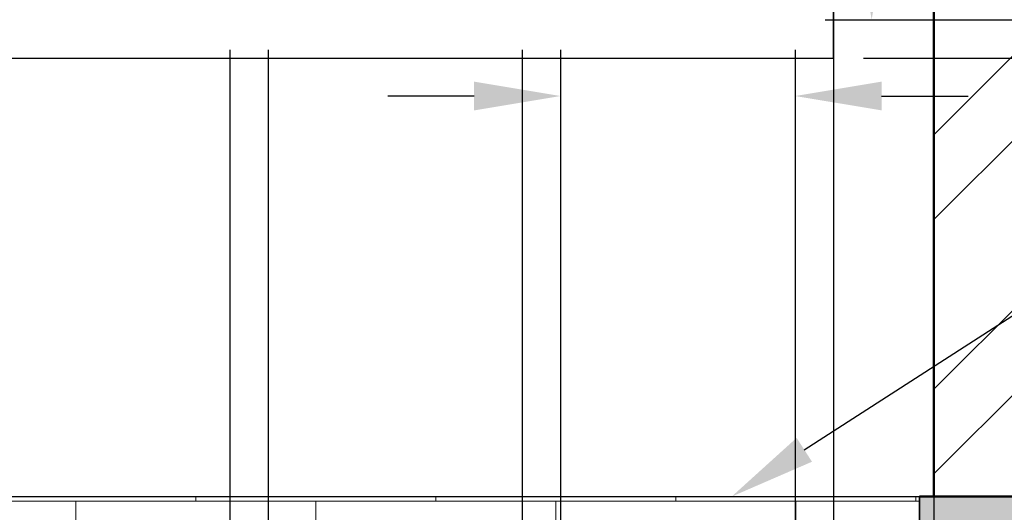
# Model space of a CAD drawing. Units: metres. Extents: x 22.1 to 34.4, y 4.4 to 12.4.
# Tile 5 of 8: x 29.6 to 31.7, y 8.5 to 9.5. Entities that reach past the tile are written whole.
import ezdxf
from ezdxf import colors
from ezdxf.entities.mleader import LeaderData, LeaderLine
from ezdxf.math import Vec2, Vec3

# ---------------------------------------------------------------- set-up
doc = ezdxf.new("R2010")
doc.units = ezdxf.units.M
doc.header["$MEASUREMENT"] = 0
for name, color, linetype, lineweight in [('A-ANNO-DIMS', 2, 'Continuous', 18), ('A-ANNO-TEXT', 7, 'Continuous', 18), ('A-FLOR', 3, 'Continuous', 25), ('A-FLOR-PATT', 252, 'Continuous', 13), ('A-GLAZ', 4, 'Continuous', 25), ('A-WALL', 7, 'Continuous', 50), ('A-WALL-PATT', 8, 'Continuous', 18), ('S-FNDN', 1, 'Continuous', 35), ('S-SLAB-PATT', 8, 'Continuous', 13)]:
    doc.layers.add(name, color=color, linetype=linetype, lineweight=lineweight)
doc.styles.get("Standard").update_dxf_attribs({"font": 'arial.ttf'})
doc.dimstyles.get("Standard").update_dxf_attribs({"dimtxt": 0.18, "dimasz": 0.18, "dimexe": 0.18, "dimexo": 0.0625, "dimgap": 0.09, "dimtad": 0, "dimtih": 1, "dimtoh": 1, "dimzin": 0, "dimdsep": 46, "dimtxsty": 'Standard', "dimcen": 0.09, "dimadec": 0, "dimazin": 0, "dimtfac": 1, "dimtofl": 0, "dimtmove": 0, "dimatfit": 3, "dimfxl": 1, "dimtolj": 1, "dimtzin": 0, "dimarcsym": 0})

# ---------------------------------------------------------------- blocks, each defined once
blk = doc.blocks.new('*D18')
at = {"layer": 'A-ANNO-DIMS', "color": 0, "lineweight": -2, "transparency": 16777216}
for p, q in [((31.3118, 10.5649), (31.5885, 10.5649)), ((31.4085, 10.3849), (31.4085, 10.2175)), ((31.4085, 9.6839), (31.4085, 9.8513)), ((31.3118, 9.5039), (31.5885, 9.5039))]:
    blk.add_line(p, q, dxfattribs=at)
at = {"layer": 'A-ANNO-DIMS', "color": 0, "transparency": 16777216}
for points in [[(31.3785, 10.3849), (31.4385, 10.3849), (31.4085, 10.5649)], [(31.3785, 9.6839), (31.4385, 9.6839), (31.4085, 9.5039)]]:
    blk.add_solid(points, dxfattribs=at)
at = {"layer": 'Defpoints', "color": 0, "transparency": 16777216}
for p in [(31.2493, 10.5649), (31.4085, 10.5649), (31.2493, 9.5039)]:
    blk.add_point(p, dxfattribs=at)
at = {"layer": 'A-ANNO-DIMS', "color": 0, "transparency": 16777216, "insert": (31.4085, 10.0344), "char_height": 0.18, "attachment_point": 5}
blk.add_mtext('\\A1;WINDOW PANE 490 1.06 TYP.', dxfattribs=at)
blk = doc.blocks.new('*D19')
at = {"layer": 'A-ANNO-DIMS', "color": 0, "lineweight": -2, "transparency": 16777216}
for p, q in [((30.7603, 9.4414), (30.7603, 9.1648)), ((31.2493, 9.4414), (31.2493, 9.1648)), ((30.5803, 9.3448), (30.4003, 9.3448)), ((31.4293, 9.3448), (31.6093, 9.3448))]:
    blk.add_line(p, q, dxfattribs=at)
at = {"layer": 'A-ANNO-DIMS', "color": 0, "transparency": 16777216}
for points in [[(30.5803, 9.3748), (30.5803, 9.3148), (30.7603, 9.3448)], [(31.4293, 9.3748), (31.4293, 9.3148), (31.2493, 9.3448)]]:
    blk.add_solid(points, dxfattribs=at)
at = {"layer": 'Defpoints', "color": 0, "transparency": 16777216}
for p in [(30.7603, 9.5039), (31.2493, 9.5039), (31.2493, 9.3448)]:
    blk.add_point(p, dxfattribs=at)
at = {"layer": 'A-ANNO-DIMS', "color": 0, "transparency": 16777216, "insert": (32.2423, 9.3448), "char_height": 0.18, "attachment_point": 5}
blk.add_mtext('\\A1;0.49 TYP.', dxfattribs=at)
blk = doc.blocks.new('*D20')
at = {"layer": 'A-ANNO-DIMS', "color": 0, "lineweight": -2, "transparency": 16777216}
for p, q in [((29.4798, 10.5649), (29.2032, 10.5649)), ((29.3832, 10.3849), (29.3832, 10.2176)), ((29.3832, 9.6839), (29.3832, 9.8512)), ((29.4798, 9.5039), (29.2032, 9.5039))]:
    blk.add_line(p, q, dxfattribs=at)
at = {"layer": 'A-ANNO-DIMS', "color": 0, "transparency": 16777216}
for points in [[(29.3532, 10.3849), (29.4132, 10.3849), (29.3832, 10.5649)], [(29.3532, 9.6839), (29.4132, 9.6839), (29.3832, 9.5039)]]:
    blk.add_solid(points, dxfattribs=at)
at = {"layer": 'Defpoints', "color": 0, "transparency": 16777216}
for p in [(29.3832, 10.5649), (29.5423, 10.5649), (29.5423, 9.5039)]:
    blk.add_point(p, dxfattribs=at)
at = {"layer": 'A-ANNO-DIMS', "color": 0, "transparency": 16777216, "insert": (29.3832, 10.0344), "char_height": 0.18, "attachment_point": 5}
blk.add_mtext('\\A1;WINDOW PANE 530 1.06 TYP.', dxfattribs=at)
blk = doc.blocks.new('*D23')
at = {"layer": 'A-ANNO-DIMS', "color": 0, "lineweight": -2, "transparency": 16777216}
for p, q in [((28.0901, 11.4474), (28.0901, 6.2449)), ((31.5381, 11.4474), (31.5381, 6.2449)), ((28.2701, 6.4249), (29.4202, 6.4249)), ((31.3581, 6.4249), (30.2079, 6.4249))]:
    blk.add_line(p, q, dxfattribs=at)
at = {"layer": 'A-ANNO-DIMS', "color": 0, "transparency": 16777216}
for points in [[(28.2701, 6.4549), (28.2701, 6.3949), (28.0901, 6.4249)], [(31.3581, 6.4549), (31.3581, 6.3949), (31.5381, 6.4249)]]:
    blk.add_solid(points, dxfattribs=at)
at = {"layer": 'Defpoints', "color": 0, "transparency": 16777216}
for p in [(28.0901, 11.5099), (31.5381, 11.5099), (31.5381, 6.4249)]:
    blk.add_point(p, dxfattribs=at)
at = {"layer": 'A-ANNO-DIMS', "color": 0, "transparency": 16777216, "insert": (29.8141, 6.4249), "char_height": 0.18, "attachment_point": 5}
blk.add_mtext('\\A1;3.448', dxfattribs=at)
blk = doc.blocks.new('*D27')
at = {"layer": 'A-ANNO-DIMS', "color": 0, "lineweight": -2, "transparency": 16777216}
for p, q in [((31.5381, 11.4474), (31.5381, 6.2449)), ((31.7781, 11.4474), (31.7781, 6.2449)), ((31.3581, 6.4249), (31.1781, 6.4249)), ((31.9581, 6.4249), (32.1381, 6.4249))]:
    blk.add_line(p, q, dxfattribs=at)
at = {"layer": 'A-ANNO-DIMS', "color": 0, "transparency": 16777216}
for points in [[(31.3581, 6.4549), (31.3581, 6.3949), (31.5381, 6.4249)], [(31.9581, 6.4549), (31.9581, 6.3949), (31.7781, 6.4249)]]:
    blk.add_solid(points, dxfattribs=at)
at = {"layer": 'Defpoints', "color": 0, "transparency": 16777216}
for p in [(31.5381, 11.5099), (31.7781, 11.5099), (31.7781, 6.4249)]:
    blk.add_point(p, dxfattribs=at)
at = {"layer": 'A-ANNO-DIMS', "color": 0, "transparency": 16777216, "insert": (32.4615, 6.4249), "char_height": 0.18, "attachment_point": 5}
blk.add_mtext('\\A1;0.24', dxfattribs=at)
blk = doc.blocks.new('*D28')
at = {"layer": 'A-ANNO-DIMS', "color": 0, "lineweight": -2, "transparency": 16777216}
for p, q in [((31.7781, 11.4474), (31.7781, 6.2449)), ((31.9781, 11.4474), (31.9781, 6.2449)), ((31.5981, 6.4249), (31.4181, 6.4249)), ((32.1581, 6.4249), (32.3381, 6.4249))]:
    blk.add_line(p, q, dxfattribs=at)
at = {"layer": 'A-ANNO-DIMS', "color": 0, "transparency": 16777216}
for points in [[(31.5981, 6.4549), (31.5981, 6.3949), (31.7781, 6.4249)], [(32.1581, 6.4549), (32.1581, 6.3949), (31.9781, 6.4249)]]:
    blk.add_solid(points, dxfattribs=at)
at = {"layer": 'Defpoints', "color": 0, "transparency": 16777216}
for p in [(31.7781, 11.5099), (31.9781, 11.5099), (31.9781, 6.4249)]:
    blk.add_point(p, dxfattribs=at)
at = {"layer": 'A-ANNO-DIMS', "color": 0, "transparency": 16777216, "insert": (32.6615, 6.4249), "char_height": 0.18, "attachment_point": 5}
blk.add_mtext('\\A1;0.20', dxfattribs=at)
blk = doc.blocks.new('*D33')
at = {"layer": 'A-ANNO-DIMS', "color": 0, "lineweight": -2, "transparency": 16777216}
for p, q in [((31.5381, 11.4474), (31.5381, 6.2449)), ((31.3293, 10.5774), (31.3293, 6.2449)), ((31.1493, 6.4249), (30.9693, 6.4249)), ((31.7181, 6.4249), (31.8981, 6.4249))]:
    blk.add_line(p, q, dxfattribs=at)
at = {"layer": 'A-ANNO-DIMS', "color": 0, "transparency": 16777216}
for points in [[(31.1493, 6.4549), (31.1493, 6.3949), (31.3293, 6.4249)], [(31.7181, 6.4549), (31.7181, 6.3949), (31.5381, 6.4249)]]:
    blk.add_solid(points, dxfattribs=at)
at = {"layer": 'Defpoints', "color": 0, "transparency": 16777216}
for p in [(31.5381, 11.5099), (31.3293, 10.6399), (31.5381, 6.4249)]:
    blk.add_point(p, dxfattribs=at)
at = {"layer": 'A-ANNO-DIMS', "color": 0, "transparency": 16777216, "insert": (32.2045, 6.4249), "char_height": 0.18, "attachment_point": 5}
blk.add_mtext('\\A1;0.21', dxfattribs=at)
blk = doc.blocks.new('*D34')
at = {"layer": 'A-ANNO-DIMS', "color": 0, "lineweight": -2, "transparency": 16777216}
for p, q in [((28.8933, 9.3614), (28.8933, 6.2449)), ((31.3293, 9.3614), (31.3293, 6.2449)), ((29.0733, 6.4249), (29.7162, 6.4249)), ((31.1493, 6.4249), (30.5065, 6.4249))]:
    blk.add_line(p, q, dxfattribs=at)
at = {"layer": 'A-ANNO-DIMS', "color": 0, "transparency": 16777216}
for points in [[(29.0733, 6.4549), (29.0733, 6.3949), (28.8933, 6.4249)], [(31.1493, 6.4549), (31.1493, 6.3949), (31.3293, 6.4249)]]:
    blk.add_solid(points, dxfattribs=at)
at = {"layer": 'Defpoints', "color": 0, "transparency": 16777216}
for p in [(28.8933, 9.4239), (31.3293, 9.4239), (31.3293, 6.4249)]:
    blk.add_point(p, dxfattribs=at)
at = {"layer": 'A-ANNO-DIMS', "color": 0, "transparency": 16777216, "insert": (30.1113, 6.4249), "char_height": 0.18, "attachment_point": 5}
blk.add_mtext('\\A1;2.436', dxfattribs=at)
blk = doc.blocks.new('*D35')
at = {"layer": 'A-ANNO-DIMS', "color": 0, "lineweight": -2, "transparency": 16777216}
for p, q in [((28.9733, 9.4414), (28.9733, 6.2449)), ((28.8933, 9.3614), (28.8933, 6.2449)), ((28.7133, 6.4249), (28.5333, 6.4249)), ((29.1533, 6.4249), (29.3333, 6.4249))]:
    blk.add_line(p, q, dxfattribs=at)
at = {"layer": 'A-ANNO-DIMS', "color": 0, "transparency": 16777216}
for points in [[(28.7133, 6.4549), (28.7133, 6.3949), (28.8933, 6.4249)], [(29.1533, 6.4549), (29.1533, 6.3949), (28.9733, 6.4249)]]:
    blk.add_solid(points, dxfattribs=at)
at = {"layer": 'Defpoints', "color": 0, "transparency": 16777216}
for p in [(28.9733, 9.5039), (28.8933, 9.4239), (28.9733, 6.4249)]:
    blk.add_point(p, dxfattribs=at)
at = {"layer": 'A-ANNO-DIMS', "color": 0, "transparency": 16777216, "insert": (29.6573, 6.4249), "char_height": 0.18, "attachment_point": 5}
blk.add_mtext('\\A1;0.08', dxfattribs=at)
blk = doc.blocks.new('*D36')
at = {"layer": 'A-ANNO-DIMS', "color": 0, "lineweight": -2, "transparency": 16777216}
for p, q in [((29.4623, 9.4414), (29.4623, 6.2449)), ((29.5423, 9.4414), (29.5423, 6.2449)), ((29.2823, 6.4249), (29.1023, 6.4249)), ((29.7223, 6.4249), (29.9023, 6.4249))]:
    blk.add_line(p, q, dxfattribs=at)
at = {"layer": 'A-ANNO-DIMS', "color": 0, "transparency": 16777216}
for points in [[(29.2823, 6.4549), (29.2823, 6.3949), (29.4623, 6.4249)], [(29.7223, 6.4549), (29.7223, 6.3949), (29.5423, 6.4249)]]:
    blk.add_solid(points, dxfattribs=at)
at = {"layer": 'Defpoints', "color": 0, "transparency": 16777216}
for p in [(29.4623, 9.5039), (29.5423, 9.5039), (29.5423, 6.4249)]:
    blk.add_point(p, dxfattribs=at)
at = {"layer": 'A-ANNO-DIMS', "color": 0, "transparency": 16777216, "insert": (30.2263, 6.4249), "char_height": 0.18, "attachment_point": 5}
blk.add_mtext('\\A1;0.08', dxfattribs=at)
blk = doc.blocks.new('*D37')
at = {"layer": 'A-ANNO-DIMS', "color": 0, "lineweight": -2, "transparency": 16777216}
for p, q in [((30.0713, 9.4414), (30.0713, 6.2449)), ((30.1513, 9.4414), (30.1513, 6.2449)), ((29.8913, 6.4249), (29.7113, 6.4249)), ((30.3313, 6.4249), (30.5113, 6.4249))]:
    blk.add_line(p, q, dxfattribs=at)
at = {"layer": 'A-ANNO-DIMS', "color": 0, "transparency": 16777216}
for points in [[(29.8913, 6.4549), (29.8913, 6.3949), (30.0713, 6.4249)], [(30.3313, 6.4549), (30.3313, 6.3949), (30.1513, 6.4249)]]:
    blk.add_solid(points, dxfattribs=at)
at = {"layer": 'Defpoints', "color": 0, "transparency": 16777216}
for p in [(30.0713, 9.5039), (30.1513, 9.5039), (30.1513, 6.4249)]:
    blk.add_point(p, dxfattribs=at)
at = {"layer": 'A-ANNO-DIMS', "color": 0, "transparency": 16777216, "insert": (30.8353, 6.4249), "char_height": 0.18, "attachment_point": 5}
blk.add_mtext('\\A1;0.08', dxfattribs=at)
blk = doc.blocks.new('*D38')
at = {"layer": 'A-ANNO-DIMS', "color": 0, "lineweight": -2, "transparency": 16777216}
for p, q in [((30.6803, 9.4414), (30.6803, 6.2449)), ((30.7603, 9.4414), (30.7603, 6.2449)), ((30.5003, 6.4249), (30.3203, 6.4249)), ((30.9403, 6.4249), (31.1203, 6.4249))]:
    blk.add_line(p, q, dxfattribs=at)
at = {"layer": 'A-ANNO-DIMS', "color": 0, "transparency": 16777216}
for points in [[(30.5003, 6.4549), (30.5003, 6.3949), (30.6803, 6.4249)], [(30.9403, 6.4549), (30.9403, 6.3949), (30.7603, 6.4249)]]:
    blk.add_solid(points, dxfattribs=at)
at = {"layer": 'Defpoints', "color": 0, "transparency": 16777216}
for p in [(30.6803, 9.5039), (30.7603, 9.5039), (30.7603, 6.4249)]:
    blk.add_point(p, dxfattribs=at)
at = {"layer": 'A-ANNO-DIMS', "color": 0, "transparency": 16777216, "insert": (31.4443, 6.4249), "char_height": 0.18, "attachment_point": 5}
blk.add_mtext('\\A1;0.08', dxfattribs=at)
blk = doc.blocks.new('*D39')
at = {"layer": 'A-ANNO-DIMS', "color": 0, "lineweight": -2, "transparency": 16777216}
for p, q in [((31.2493, 9.4414), (31.2493, 6.2449)), ((31.3293, 9.3614), (31.3293, 6.2449)), ((31.0693, 6.4249), (30.8893, 6.4249)), ((31.5093, 6.4249), (31.6893, 6.4249))]:
    blk.add_line(p, q, dxfattribs=at)
at = {"layer": 'A-ANNO-DIMS', "color": 0, "transparency": 16777216}
for points in [[(31.0693, 6.4549), (31.0693, 6.3949), (31.2493, 6.4249)], [(31.5093, 6.4549), (31.5093, 6.3949), (31.3293, 6.4249)]]:
    blk.add_solid(points, dxfattribs=at)
at = {"layer": 'Defpoints', "color": 0, "transparency": 16777216}
for p in [(31.2493, 9.5039), (31.3293, 9.4239), (31.3293, 6.4249)]:
    blk.add_point(p, dxfattribs=at)
at = {"layer": 'A-ANNO-DIMS', "color": 0, "transparency": 16777216, "insert": (32.0133, 6.4249), "char_height": 0.18, "attachment_point": 5}
blk.add_mtext('\\A1;0.08', dxfattribs=at)
blk = doc.blocks.new('*D40')
at = {"layer": 'A-ANNO-DIMS', "color": 0, "lineweight": -2, "transparency": 16777216}
for p, q in [((31.3918, 10.6399), (33.8537, 10.6399)), ((33.6737, 10.4599), (33.6737, 10.2138)), ((33.6737, 9.6039), (33.6737, 9.85)), ((31.3918, 9.4239), (33.8537, 9.4239))]:
    blk.add_line(p, q, dxfattribs=at)
at = {"layer": 'A-ANNO-DIMS', "color": 0, "transparency": 16777216}
for points in [[(33.6437, 10.4599), (33.7037, 10.4599), (33.6737, 10.6399)], [(33.6437, 9.6039), (33.7037, 9.6039), (33.6737, 9.4239)]]:
    blk.add_solid(points, dxfattribs=at)
at = {"layer": 'Defpoints', "color": 0, "transparency": 16777216}
for p in [(31.3293, 10.6399), (31.3293, 9.4239), (33.6737, 9.4239)]:
    blk.add_point(p, dxfattribs=at)
at = {"layer": 'A-ANNO-DIMS', "color": 0, "transparency": 16777216, "insert": (33.6737, 10.0319), "char_height": 0.18, "attachment_point": 5}
blk.add_mtext('\\A1;1.216', dxfattribs=at)
blk = doc.blocks.new('*D42')
at = {"layer": 'A-ANNO-DIMS', "color": 0, "lineweight": -2, "transparency": 16777216}
for p, q in [((33.6737, 9.6839), (33.6737, 9.8639)), ((33.6737, 9.8639), (33.8537, 9.8639)), ((31.3118, 9.5039), (33.8537, 9.5039)), ((31.3918, 9.4239), (33.8537, 9.4239)), ((33.6737, 9.2439), (33.6737, 9.0639))]:
    blk.add_line(p, q, dxfattribs=at)
at = {"layer": 'A-ANNO-DIMS', "color": 0, "transparency": 16777216}
for points in [[(33.6437, 9.6839), (33.7037, 9.6839), (33.6737, 9.5039)], [(33.6437, 9.2439), (33.7037, 9.2439), (33.6737, 9.4239)]]:
    blk.add_solid(points, dxfattribs=at)
at = {"layer": 'Defpoints', "color": 0, "transparency": 16777216}
for p in [(31.2493, 9.5039), (33.6737, 9.5039), (31.3293, 9.4239)]:
    blk.add_point(p, dxfattribs=at)
at = {"layer": 'A-ANNO-DIMS', "color": 0, "transparency": 16777216, "insert": (34.1776, 9.8639), "char_height": 0.18, "attachment_point": 5}
blk.add_mtext('\\A1;0.08', dxfattribs=at)
blk = doc.blocks.new('*D43')
at = {"layer": 'A-ANNO-DIMS', "color": 0, "lineweight": -2, "transparency": 16777216}
for p, q in [((31.3918, 9.4239), (33.8537, 9.4239)), ((33.6737, 9.2439), (33.6737, 9.1488)), ((33.6737, 8.6899), (33.6737, 8.785)), ((31.5706, 8.5099), (33.8537, 8.5099))]:
    blk.add_line(p, q, dxfattribs=at)
at = {"layer": 'A-ANNO-DIMS', "color": 0, "transparency": 16777216}
for points in [[(33.6437, 9.2439), (33.7037, 9.2439), (33.6737, 9.4239)], [(33.6437, 8.6899), (33.7037, 8.6899), (33.6737, 8.5099)]]:
    blk.add_solid(points, dxfattribs=at)
at = {"layer": 'Defpoints', "color": 0, "transparency": 16777216}
for p in [(31.3293, 9.4239), (31.5081, 8.5099), (33.6737, 8.5099)]:
    blk.add_point(p, dxfattribs=at)
at = {"layer": 'A-ANNO-DIMS', "color": 0, "transparency": 16777216, "insert": (33.6737, 8.9669), "char_height": 0.18, "attachment_point": 5}
blk.add_mtext('\\A1;0.914', dxfattribs=at)
blk = doc.blocks.new('*D44')
at = {"layer": 'A-ANNO-DIMS', "color": 0, "lineweight": -2, "transparency": 16777216}
for p, q in [((33.6737, 8.6899), (33.6737, 8.8699)), ((24.8474, 8.5099), (33.8537, 8.5099)), ((24.5474, 8.4099), (33.8537, 8.4099)), ((33.6737, 8.2299), (33.6737, 8.0499)), ((33.6737, 8.0499), (33.4937, 8.0499))]:
    blk.add_line(p, q, dxfattribs=at)
at = {"layer": 'A-ANNO-DIMS', "color": 0, "transparency": 16777216}
for points in [[(33.6437, 8.6899), (33.7037, 8.6899), (33.6737, 8.5099)], [(33.6437, 8.2299), (33.7037, 8.2299), (33.6737, 8.4099)]]:
    blk.add_solid(points, dxfattribs=at)
at = {"layer": 'Defpoints', "color": 0, "transparency": 16777216}
for p in [(24.7849, 8.5099), (24.4849, 8.4099), (33.6737, 8.4099)]:
    blk.add_point(p, dxfattribs=at)
at = {"layer": 'A-ANNO-DIMS', "color": 0, "transparency": 16777216, "insert": (33.1702, 8.0499), "char_height": 0.18, "attachment_point": 5}
blk.add_mtext('\\A1;0.10', dxfattribs=at)
blk = doc.blocks.new('*D45')
at = {"layer": 'A-ANNO-DIMS', "color": 0, "lineweight": -2, "transparency": 16777216}
for p, q in [((33.6737, 8.5899), (33.6737, 8.7699)), ((24.5474, 8.4099), (33.8537, 8.4099)), ((24.8474, 8.3119), (33.8537, 8.3119)), ((33.6737, 8.1319), (33.6737, 7.9519)), ((33.6737, 7.9519), (33.4937, 7.9519))]:
    blk.add_line(p, q, dxfattribs=at)
at = {"layer": 'A-ANNO-DIMS', "color": 0, "transparency": 16777216}
for points in [[(33.6437, 8.5899), (33.7037, 8.5899), (33.6737, 8.4099)], [(33.6437, 8.1319), (33.7037, 8.1319), (33.6737, 8.3119)]]:
    blk.add_solid(points, dxfattribs=at)
at = {"layer": 'Defpoints', "color": 0, "transparency": 16777216}
for p in [(24.4849, 8.4099), (24.7849, 8.3119), (33.6737, 8.3119)]:
    blk.add_point(p, dxfattribs=at)
at = {"layer": 'A-ANNO-DIMS', "color": 0, "transparency": 16777216, "insert": (33.0998, 7.9519), "char_height": 0.18, "attachment_point": 5}
blk.add_mtext('\\A1;0.098', dxfattribs=at)
blk = doc.blocks.new('*D46')
at = {"layer": 'A-ANNO-DIMS', "color": 0, "lineweight": -2, "transparency": 16777216}
for p, q in [((33.6737, 8.4919), (33.6737, 8.6719)), ((24.8474, 8.3119), (33.8537, 8.3119)), ((24.8474, 8.1578), (33.8537, 8.1578)), ((33.6737, 7.9778), (33.6737, 7.7978)), ((33.6737, 7.7978), (33.4937, 7.7978))]:
    blk.add_line(p, q, dxfattribs=at)
at = {"layer": 'A-ANNO-DIMS', "color": 0, "transparency": 16777216}
for points in [[(33.6437, 8.4919), (33.7037, 8.4919), (33.6737, 8.3119)], [(33.6437, 7.9778), (33.7037, 7.9778), (33.6737, 8.1578)]]:
    blk.add_solid(points, dxfattribs=at)
at = {"layer": 'Defpoints', "color": 0, "transparency": 16777216}
for p in [(24.7849, 8.3119), (24.7849, 8.1578), (33.6737, 8.1578)]:
    blk.add_point(p, dxfattribs=at)
at = {"layer": 'A-ANNO-DIMS', "color": 0, "transparency": 16777216, "insert": (33.1692, 7.7978), "char_height": 0.18, "attachment_point": 5}
blk.add_mtext('\\A1;0.15', dxfattribs=at)
blk = doc.blocks.new('*D47')
at = {"layer": 'A-ANNO-DIMS', "color": 0, "lineweight": -2, "transparency": 16777216}
for p, q in [((33.6737, 8.3378), (33.6737, 8.5178)), ((24.8474, 8.1578), (33.8537, 8.1578)), ((24.8474, 7.9099), (33.8537, 7.9099)), ((33.6737, 7.7299), (33.6737, 7.5499)), ((33.6737, 7.5499), (33.4937, 7.5499))]:
    blk.add_line(p, q, dxfattribs=at)
at = {"layer": 'A-ANNO-DIMS', "color": 0, "transparency": 16777216}
for points in [[(33.6437, 8.3378), (33.7037, 8.3378), (33.6737, 8.1578)], [(33.6437, 7.7299), (33.7037, 7.7299), (33.6737, 7.9099)]]:
    blk.add_solid(points, dxfattribs=at)
at = {"layer": 'Defpoints', "color": 0, "transparency": 16777216}
for p in [(24.7849, 8.1578), (24.7849, 7.9099), (33.6737, 7.9099)]:
    blk.add_point(p, dxfattribs=at)
at = {"layer": 'A-ANNO-DIMS', "color": 0, "transparency": 16777216, "insert": (33.1692, 7.5499), "char_height": 0.18, "attachment_point": 5}
blk.add_mtext('\\A1;0.25', dxfattribs=at)

msp = doc.modelspace()

# ---------------------------------------------------------------- hatches: boundary and pattern name
at = {"layer": 'A-FLOR-PATT'}
h = msp.add_hatch(dxfattribs=at)
h.set_pattern_fill('BRICK', color=256)
h.paths.add_polyline_path([(31.5081, 8.5099), (28.1201, 8.5099), (28.1201, 8.4099), (31.5081, 8.4099)])
h.paths.add_polyline_path([(27.8201, 8.5099), (27.0468, 8.5099), (26.6456, 8.5099), (26.6456, 8.4099), (27.8201, 8.4099)])
h.paths.add_polyline_path([(26.3456, 8.5099), (25.6173, 8.5099), (24.7849, 8.5099), (24.7849, 8.4099), (26.3456, 8.4099)])
at = {"layer": 'A-WALL-PATT'}
h = msp.add_hatch(dxfattribs=at)
h.set_pattern_fill('ANSI32', color=256)
h.paths.add_polyline_path([(24.7549, 11.5099), (24.5149, 11.5099), (24.5149, 11.1399), (24.7549, 11.1399)])
h.paths.add_polyline_path([(24.7549, 10.6399), (24.5149, 10.6399), (24.5149, 8.5099), (24.6349, 8.5099), (24.7549, 8.5099)])
h.paths.add_polyline_path([(26.5706, 11.5099), (26.4206, 11.5099), (26.4206, 8.5099), (26.5706, 8.5099)])
h.paths.add_polyline_path([(28.0901, 10.6399), (28.0901, 11.5099), (27.8501, 11.5099), (27.8501, 8.5099), (28.0901, 8.5099)])
h.paths.add_polyline_path([(31.7781, 11.5099), (31.5381, 11.5099), (31.5381, 8.5099), (31.6581, 8.5099), (31.7781, 8.5099)])
at = {"layer": 'S-SLAB-PATT'}
h = msp.add_hatch(dxfattribs=at)
h.set_pattern_fill('AR-CONC', color=256, scale=0.04)
h.set_pattern_definition([(50, (0, 0), (0.286904, -0.0251009), [0.03, -0.33]), (355, (0, 0), (-0.0555005, 0.3008769), [0.024, -0.264]), (100.4514, (0.0239, -0.0021), (0.2314035, 0.275776), [0.025496, -0.2804568]), (46.1842, (0, 0.08), (0.4268965, -0.0662077), [0.045, -0.495]), (96.6356, (0.03557, 0.0745), (0.373865, 0.3896474), [0.038244, -0.4206855]), (351.1842, (0, 0.08), (0.373865, 0.3896474), [0.036, -0.396]), (21, (0.04, 0.06), (0.2387628, -0.1610476), [0.03, -0.33]), (326, (0.04, 0.06), (0.0973261, 0.29006), [0.024, -0.264]), (71.4514, (0.0599, 0.04658), (0.336089, 0.1290125), [0.025496, -0.2804568]), (37.5, (0, 0), (0.00486394, 0.13315754), [0, -0.2608, 0, -0.268, 0, -0.265]), (7.5, (0, 0), (0.1052278, 0.1577647), [0, -0.1528, 0, -0.2548, 0, -0.101]), (327.5, (-0.0892, 0), (0.21352897, -0.00902195), [0, -0.1, 0, -0.312, 0, -0.414]), (317.5, (-0.1292, 0), (0.2332745, 0.040042), [0, -0.13, 0, -0.2072, 0, -0.294])])
h.paths.add_polyline_path([(31.9781, 11.6599), (24.3149, 11.6599), (24.3149, 11.5099), (24.5149, 11.5099), (31.7781, 11.5099), (31.9781, 11.5099)])
h.paths.add_polyline_path([(25.1849, 7.2099), (24.9849, 7.2099), (24.0849, 7.2099), (24.0849, 7.0099), (25.1849, 7.0099)])
h.paths.add_polyline_path([(32.2081, 7.2099), (32.0081, 7.2099), (31.1081, 7.2099), (31.1081, 7.0099), (32.2081, 7.0099)])
h.paths.add_polyline_path([(28.5201, 7.2099), (28.3201, 7.2099), (27.4201, 7.2099), (27.4201, 7.0099), (28.5201, 7.0099)])
h.paths.add_polyline_path([(24.7849, 8.5099), (24.6349, 8.5099), (24.5149, 8.5099), (24.4849, 8.5099), (24.4849, 8.4099), (24.7849, 8.4099)])
h.paths.add_polyline_path([(26.6456, 8.5099), (26.3456, 8.5099), (26.3456, 8.4099), (26.6456, 8.4099)])
h.paths.add_polyline_path([(28.1201, 8.5099), (28.0901, 8.5099), (27.8201, 8.5099), (27.8201, 8.4099), (28.1201, 8.4099)])
h.paths.add_polyline_path([(31.8081, 8.5099), (31.6581, 8.5099), (31.5381, 8.5099), (31.5081, 8.5099), (31.5081, 8.4099), (31.8081, 8.4099)])
h.paths.add_polyline_path([(26.3456, 8.3119), (24.7849, 8.3119), (24.7849, 8.1578), (26.3456, 8.1578)])
h.paths.add_polyline_path([(27.8201, 8.3119), (26.6456, 8.3119), (26.6456, 8.1578), (27.8201, 8.1578)])
h.paths.add_polyline_path([(31.5081, 8.3119), (28.1201, 8.3119), (28.1201, 8.1578), (31.5081, 8.1578)])

# ---------------------------------------------------------------- linework, layer by layer
at = {"layer": 'A-FLOR'}
msp.add_line((24.7849, 8.5099), (31.5081, 8.5099), dxfattribs=at)
at = {"layer": 'A-GLAZ'}
for p, q in [((31.3293, 9.4239), (31.3293, 10.6399)), ((28.8933, 9.4239), (31.3293, 9.4239))]:
    msp.add_line(p, q, dxfattribs=at)
at = {"layer": 'A-WALL'}
for p, q in [((31.5381, 8.5099), (31.5381, 11.5099)), ((31.5081, 8.5099), (31.6581, 8.5099)), ((31.6581, 8.5099), (31.5381, 8.5099)), ((31.8081, 8.5099), (31.6581, 8.5099)), ((31.6581, 8.5099), (31.7781, 8.5099))]:
    msp.add_line(p, q, dxfattribs=at)
at = {"layer": 'S-FNDN'}
msp.add_line((31.5081, 7.9099), (31.5081, 8.5099), dxfattribs=at)

# ---------------------------------------------------------------- dimensions: what is measured, and where the dimension line sits
at = {"layer": 'A-ANNO-DIMS'}
for base, p1, p2, override, picture, middle in [((31.5381, 6.4249), (28.0901, 11.5099), (31.5381, 11.5099), {"dimdec": 3, "dimlfac": 1, "dimrnd": 0, "dimzin": 0, "dimdsep": 46, "dimlunit": 2}, '*D23', (29.8141, 6.4249)), ((31.5381, 6.4249), (31.3293, 10.6399), (31.5381, 11.5099), {"dimdec": 2, "dimlfac": 1, "dimrnd": 0, "dimzin": 0, "dimdsep": 46, "dimlunit": 2}, '*D33', (32.2045, 6.4249)), ((31.7781, 6.4249), (31.5381, 11.5099), (31.7781, 11.5099), {"dimdec": 2, "dimlfac": 1, "dimrnd": 0, "dimzin": 0, "dimdsep": 46, "dimlunit": 2}, '*D27', (32.4615, 6.4249)), ((31.9781, 6.4249), (31.7781, 11.5099), (31.9781, 11.5099), {"dimdec": 2, "dimlfac": 1, "dimrnd": 0, "dimzin": 0, "dimdsep": 46, "dimlunit": 2}, '*D28', (32.6615, 6.4249)), ((28.9733, 6.4249), (28.8933, 9.4239), (28.9733, 9.5039), {"dimdec": 2, "dimlfac": 1, "dimrnd": 0, "dimzin": 0, "dimdsep": 46, "dimlunit": 2}, '*D35', (29.6573, 6.4249)), ((29.5423, 6.4249), (29.4623, 9.5039), (29.5423, 9.5039), {"dimdec": 2, "dimlfac": 1, "dimrnd": 0, "dimzin": 0, "dimdsep": 46, "dimlunit": 2}, '*D36', (30.2263, 6.4249)), ((30.1513, 6.4249), (30.0713, 9.5039), (30.1513, 9.5039), {"dimdec": 2, "dimlfac": 1, "dimrnd": 0, "dimzin": 0, "dimdsep": 46, "dimlunit": 2}, '*D37', (30.8353, 6.4249)), ((30.7603, 6.4249), (30.6803, 9.5039), (30.7603, 9.5039), {"dimdec": 2, "dimlfac": 1, "dimrnd": 0, "dimzin": 0, "dimdsep": 46, "dimlunit": 2}, '*D38', (31.4443, 6.4249)), ((31.3293, 6.4249), (31.2493, 9.5039), (31.3293, 9.4239), {"dimdec": 2, "dimlfac": 1, "dimrnd": 0, "dimzin": 0, "dimdsep": 46, "dimlunit": 2}, '*D39', (32.0133, 6.4249)), ((31.3293, 6.4249), (28.8933, 9.4239), (31.3293, 9.4239), {"dimdec": 3, "dimlfac": 1, "dimrnd": 0, "dimzin": 0, "dimdsep": 46, "dimlunit": 2}, '*D34', (30.1113, 6.4249))]:
    dim = msp.add_linear_dim(base=base, p1=p1, p2=p2, dimstyle='Standard', override=override, dxfattribs=at)
    dim.commit()
    dim.dimension.update_dxf_attribs({"geometry": picture, "text_midpoint": middle})
for base, p1, p2, text, picture, middle in [((29.3832, 10.5649), (29.5423, 9.5039), (29.5423, 10.5649), 'WINDOW PANE 530 <> TYP.', '*D20', (29.3832, 10.0344)), ((31.4085, 10.5649), (31.2493, 9.5039), (31.2493, 10.5649), 'WINDOW PANE 490 <> TYP.', '*D18', (31.4085, 10.0344))]:
    dim = msp.add_linear_dim(base=base, p1=p1, p2=p2, angle=90, text=text, dimstyle='Standard', override={"dimdec": 2, "dimrnd": 0, "dimzin": 0, "dimlunit": 2}, dxfattribs=at)
    dim.commit()
    dim.dimension.update_dxf_attribs({"geometry": picture, "text_midpoint": middle})
for base, p1, p2, override, picture, middle in [((33.6737, 9.4239), (31.3293, 10.6399), (31.3293, 9.4239), {"dimdec": 3, "dimlfac": 1, "dimrnd": 0, "dimzin": 0, "dimdsep": 46, "dimlunit": 2}, '*D40', (33.6737, 10.0319)), ((33.6737, 9.5039), (31.3293, 9.4239), (31.2493, 9.5039), {"dimdec": 2, "dimlfac": 1, "dimrnd": 0, "dimzin": 0, "dimdsep": 46, "dimlunit": 2}, '*D42', (34.1776, 9.8639)), ((33.6737, 8.5099), (31.3293, 9.4239), (31.5081, 8.5099), {"dimdec": 3, "dimlfac": 1, "dimrnd": 0, "dimzin": 0, "dimdsep": 46, "dimlunit": 2}, '*D43', (33.6737, 8.9669)), ((33.6737, 8.4099), (24.7849, 8.5099), (24.4849, 8.4099), {"dimdec": 2, "dimlfac": 1, "dimrnd": 0, "dimzin": 0, "dimdsep": 46, "dimlunit": 2}, '*D44', (33.1702, 8.0499)), ((33.6737, 8.3119), (24.4849, 8.4099), (24.7849, 8.3119), {"dimdec": 3, "dimlfac": 1, "dimrnd": 0, "dimzin": 0, "dimdsep": 46, "dimlunit": 2}, '*D45', (33.0998, 7.9519)), ((33.6737, 8.1578), (24.7849, 8.3119), (24.7849, 8.1578), {"dimdec": 2, "dimlfac": 1, "dimrnd": 0, "dimzin": 0, "dimdsep": 46, "dimlunit": 2}, '*D46', (33.1692, 7.7978)), ((33.6737, 7.9099), (24.7849, 8.1578), (24.7849, 7.9099), {"dimdec": 2, "dimlfac": 1, "dimrnd": 0, "dimzin": 0, "dimdsep": 46, "dimlunit": 2}, '*D47', (33.1692, 7.5499))]:
    dim = msp.add_linear_dim(base=base, p1=p1, p2=p2, angle=90, dimstyle='Standard', override=override, dxfattribs=at)
    dim.commit()
    dim.dimension.update_dxf_attribs({"geometry": picture, "text_midpoint": middle})
dim = msp.add_linear_dim(base=(31.2493, 9.3448), p1=(30.7603, 9.5039), p2=(31.2493, 9.5039), text='<> TYP.', dimstyle='Standard', override={"dimdec": 2, "dimrnd": 0, "dimzin": 0, "dimlunit": 2}, dxfattribs=at)
dim.commit()
dim.dimension.update_dxf_attribs({"geometry": '*D19', "text_midpoint": (32.2423, 9.3448)})

# ---------------------------------------------------------------- leaders
at = {"layer": 'A-ANNO-TEXT'}
ml = msp.add_multileader_mtext('Standard', dxfattribs=at)
ml.set_content('Tiles', color=256)
ml.set_leader_properties()
ml.build(insert=Vec2(0, 0))
ml.multileader.update_dxf_attribs({"dogleg_length": 0.36, "arrow_head_size": 0.18})
ctx = ml.context
ctx.base_point, ctx.char_height, ctx.arrow_head_size, ctx.landing_gap_size, ctx.plane_origin = Vec3(32.1951, 9.0617), 0.18, 0.18, 0.09, Vec3(31.1169, 8.5099)
notes = []
notes.append((ctx, [(0, (1, 1, 0), (31.9729, 9.0617), (1, 0), 0.2223, [(0, [(31.1169, 8.5099)], 0, [])])]))
ctx.mtext.insert, ctx.mtext.flow_direction = Vec3(32.2851, 9.1532), 5
for ctx, leaders in notes:
    for number, flags, end, landing, length, lines in leaders:
        leader = LeaderData()
        leader.index, (leader.has_last_leader_line, leader.has_dogleg_vector, leader.attachment_direction) = number, flags
        leader.last_leader_point, leader.dogleg_vector, leader.dogleg_length = Vec3(end), Vec3(landing), length
        for number, points, colour, breaks in lines:
            line = LeaderLine()
            line.index, line.vertices, line.color, line.breaks = number, Vec3.list(points), colors.encode_raw_color(colour), breaks
            leader.lines.append(line)
        ctx.leaders.append(leader)

doc.saveas('drawing.dxf')
